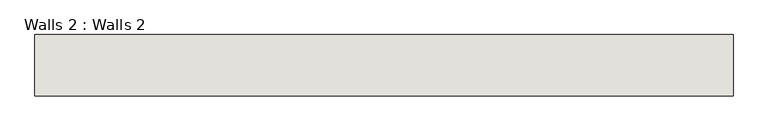
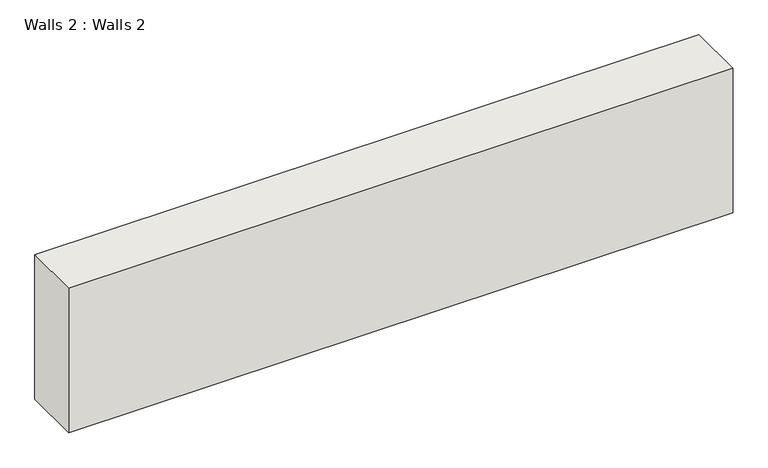
"""IFC4 building model written with IfcOpenShell, lengths in millimetres: wall geometry, Walls 2 : Walls 2."""

from ifc_helpers import new_model, si_unit, frame, origin, place, context, project, spatial, polyline, outline, extrude, source, transform, mapped, element, save


def walls_2_walls_2_a0716ef0(model_context):
    return source(origin(), model_context, "Body", "SweptSolid", [
        extrude(outline(polyline([(-1482.6998814, 272.7610824), (-5851.4998814, 272.7610824), (-5851.4998814, 656.4749382), (-1482.6998814, 656.4749382), (-1482.6998814, 272.7610824)])), frame((0.0, 0.0, 10599.4380846), z_axis=(0.0, 0.0, 1.0), x_axis=(1.0, 0.0, 0.0)), (0.0, 0.0, 1.0), 1003.8673686),
    ])


if __name__ == "__main__":
    model = new_model("IFC4")
    model_context = context("Model", 3, world=origin())
    ifc_project = project(units=[si_unit("LENGTHUNIT", "METRE", prefix="MILLI")], contexts=[model_context])
    site = spatial("IfcSite", under=ifc_project)
    building = spatial("IfcBuilding", under=site)
    placement = place(None, origin())
    walls_2_walls_2_shape = walls_2_walls_2_a0716ef0(model_context)
    element("IfcWall", 1, ObjectType="Walls 2 : Walls 2", at=placement, inside=building, context=model_context, shape_type="MappedRepresentation", body=[
        mapped(walls_2_walls_2_shape, transform((0.0, 0.0, 0.0), x_axis=(1.0, 0.0, 0.0), y_axis=(0.0, 1.0, 0.0), z_axis=(0.0, 0.0, 1.0))),
    ])
    save(model, "model.ifc")

# Revit data of these elements
# Element 1 (IfcWall, "Walls 2 : Walls 2")
#   Materials on its faces: "Default Wall"
# Materials
#   "Default Wall": colour RGB 128 128 128, transparency 0
